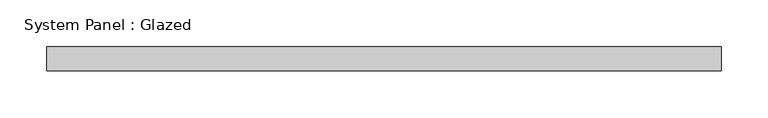
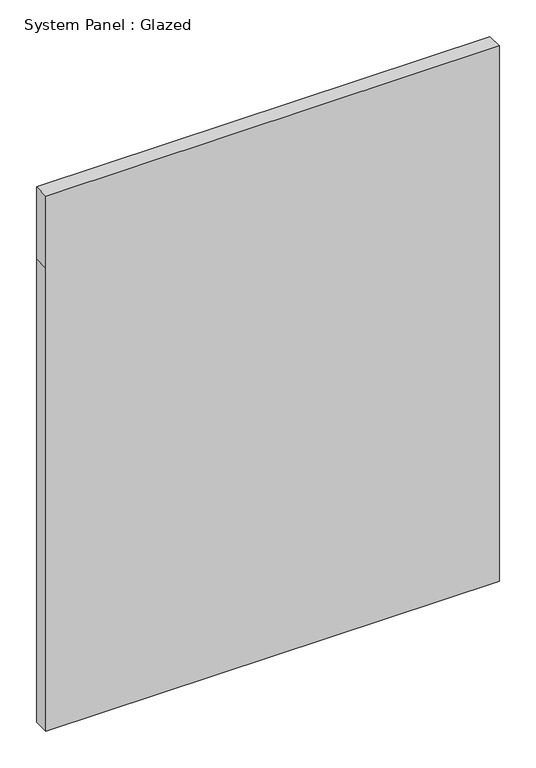
"""IFC4 building model written with IfcOpenShell, lengths in millimetres: plate geometry, System Panel : Glazed."""

from ifc_helpers import new_model, si_unit, frame, origin, place, context, project, spatial, polyline, outline, extrude, source, transform, mapped, element, save


def system_panel_glazed_4b08eeb4(model_context):
    return source(origin(), model_context, "Body", "SweptSolid", [
        extrude(outline(polyline([(0.0, -358.775), (0.0, 358.775), (774.3574877, 358.775), (895.0074877, 358.775), (895.0074877, -358.775), (774.3574877, -358.775), (0.0, -358.775)])), frame((0.0, 19.05, 0.0), z_axis=(0.0, 1.0, 0.0), x_axis=(0.0, 0.0, 1.0)), (0.0, 0.0, 1.0), 25.4),
    ])


if __name__ == "__main__":
    model = new_model("IFC4")
    model_context = context("Model", 3, world=origin())
    ifc_project = project(units=[si_unit("LENGTHUNIT", "METRE", prefix="MILLI")], contexts=[model_context])
    site = spatial("IfcSite", under=ifc_project)
    building = spatial("IfcBuilding", under=site)
    placement = place(None, origin())
    system_panel_glazed_shape = system_panel_glazed_4b08eeb4(model_context)
    element("IfcPlate", 1, ObjectType="System Panel : Glazed", at=placement, inside=building, context=model_context, shape_type="MappedRepresentation", body=[
        mapped(system_panel_glazed_shape, transform((0.0, 0.0, 0.0), x_axis=(1.0, 0.0, 0.0), y_axis=(0.0, 1.0, 0.0), z_axis=(0.0, 0.0, 1.0))),
    ])
    save(model, "model.ifc")

# Revit data of these elements
# Type "System Panel : Glazed"
#   Construction Type Id = "GSP4R"
#   Analytic Construction = "1/8 in Pilkington single glazing"
#   Visual Light Transmittance = 0.9
#   Solar Heat Gain Coefficient = 0.86
#   Heat Transfer Coefficient (U) = 1.18115 BTU/(h·ft²·°F)
#   Define Thermal Properties by = 1
# Element 1 (IfcPlate, "System Panel : Glazed")
#   Materials on its faces: "Glass"
# Materials
#   "Glass": class "Glass", colour RGB 0 128 192, transparency 0.75, Description = "Soda Lime Glass", Cost = 0
